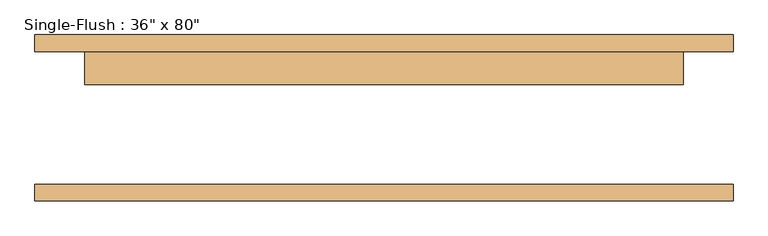
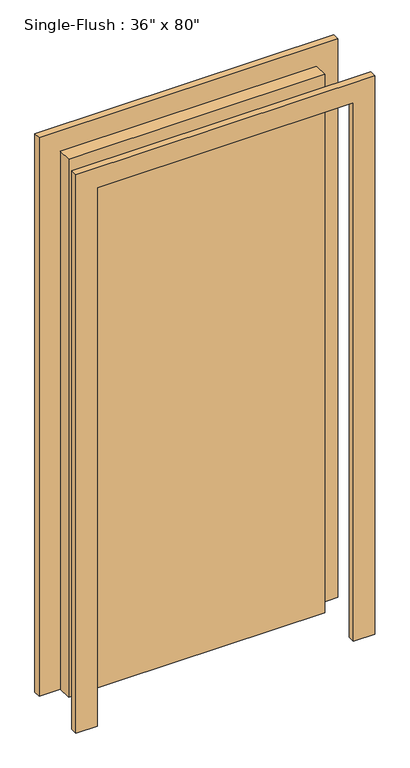
"""IFC4 building model written with IfcOpenShell, lengths in millimetres: door geometry."""

from ifc_helpers import new_model, si_unit, frame, origin, origin_with_axes, place, context, project, spatial, polyline, outline, extrude, source, transform, mapped, element, save


def door_4f2f89b6(model_context):
    return source(origin(), model_context, "Body", "SweptSolid", [
        extrude(outline(polyline([(2108.2, -533.4), (0.0, -533.4), (0.0, -457.2), (2032.0, -457.2), (2032.0, 457.2), (0.0, 457.2), (0.0, 533.4), (2108.2, 533.4), (2108.2, -533.4)])), frame((0.0, 101.6, 0.0), z_axis=(0.0, 1.0, 0.0), x_axis=(0.0, 0.0, 1.0)), (0.0, 0.0, 1.0), 25.4),
        extrude(outline(polyline([(2108.2, 533.4), (2108.2, -533.4), (0.0, -533.4), (0.0, -457.2), (2032.0, -457.2), (2032.0, 457.2), (0.0, 457.2), (0.0, 533.4), (2108.2, 533.4)])), frame((0.0, -127.0, 0.0), z_axis=(0.0, 1.0, 0.0), x_axis=(0.0, 0.0, 1.0)), (0.0, 0.0, 1.0), 25.4),
        extrude(outline(polyline([(457.2, 50.8), (-457.2, 50.8), (-457.2, 101.6), (457.2, 101.6), (457.2, 50.8)])), origin_with_axes(), (0.0, 0.0, 1.0), 2032.0),
    ])


if __name__ == "__main__":
    model = new_model("IFC4")
    model_context = context("Model", 3, world=origin())
    ifc_project = project(units=[si_unit("LENGTHUNIT", "METRE", prefix="MILLI")], contexts=[model_context])
    site = spatial("IfcSite", under=ifc_project)
    building = spatial("IfcBuilding", under=site)
    placement = place(None, origin())
    door_shape = door_4f2f89b6(model_context)
    element("IfcDoor", 1, ObjectType="Single-Flush : 36\" x 80\"", at=placement, inside=building, context=model_context, shape_type="MappedRepresentation", body=[
        mapped(door_shape, transform((0.0, 0.0, 0.0), x_axis=(1.0, 0.0, 0.0), y_axis=(0.0, 1.0, 0.0), z_axis=(0.0, 0.0, 1.0))),
    ])
    save(model, "model.ifc")

# Revit data of these elements
# Type "Single-Flush : 36\" x 80\""
#   Type Mark = "6"
#   Construction Type Id = "MDOOR"
#   Assembly Code = "C1020"
#   Analytic Construction = "Metal"
#   Thickness = 0' - 2"
#   Heat Transfer Coefficient (U) = 0.651978 BTU/(h·ft²·°F)
#   Height = 6' - 8"
#   Trim Projection Ext = 0' - 1"
#   Trim Projection Int = 0' - 1"
#   Trim Width = 0' - 3"
#   Width = 3' - 0"
#   Define Thermal Properties by = 1
#   Door Material = Door - Panel
#   Frame Material = Door - Frame
#   Visual Light Transmittance = 0
#   Solar Heat Gain Coefficient = 0
#   Function = (empty or 0)
#   Wall Closure = (empty or 0)
# Element 1 (IfcDoor, "Single-Flush : 36\" x 80\"")
#   Materials on its faces: "Door - Frame", "Door - Panel"
# Materials
#   "Door - Panel": class "Wood", colour RGB 210 159 95, transparency 0
#   "Door - Frame": colour RGB 118 70 51, transparency 0
